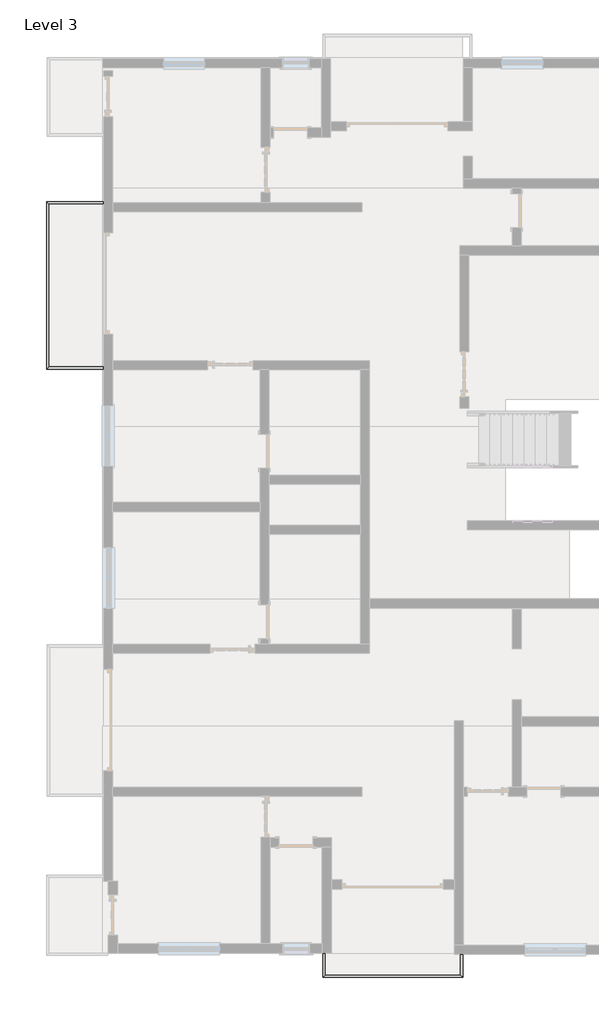
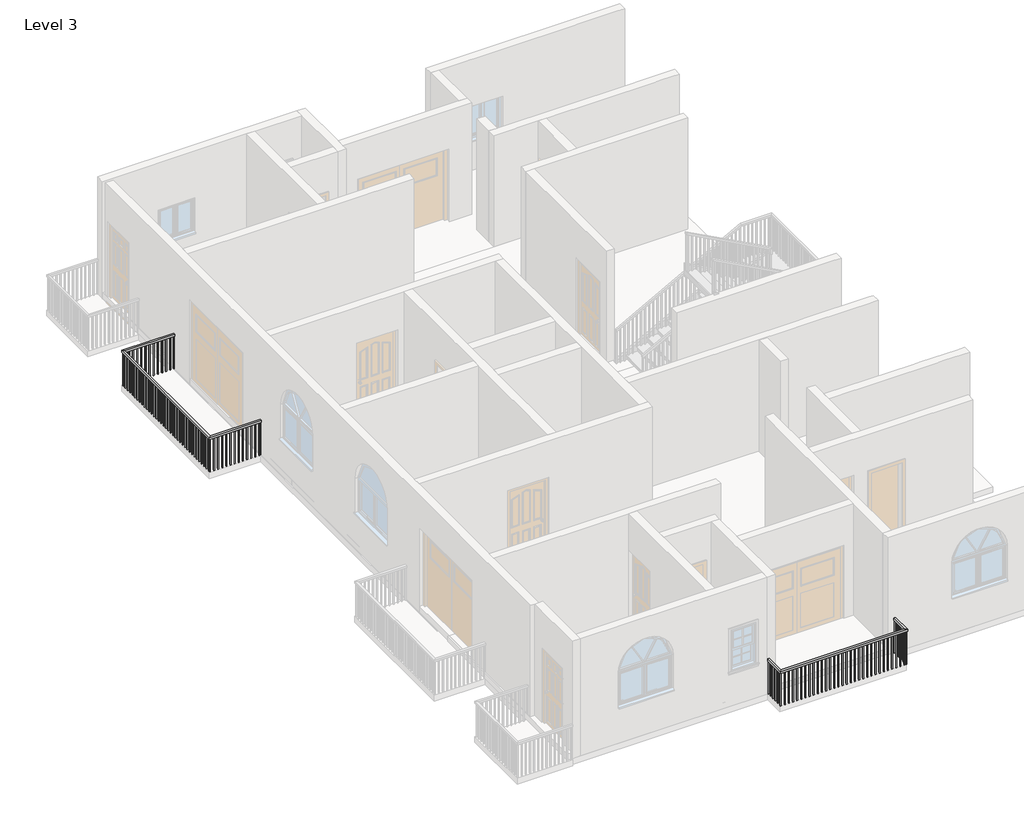
# One storey, part 4 of 7: 2 railings.
"""IFC4 building model written with IfcOpenShell, lengths in millimetres."""

from ifc_helpers import new_model, si_unit, frame, origin, place, context, project, spatial, polyline, outline, extrude, faceted_brep, element, save

model = new_model("IFC4")

# Units and contexts
model_context = context("Model", 3, world=origin())
ifc_project = project(units=[si_unit("LENGTHUNIT", "METRE", prefix="MILLI")], contexts=[model_context])

# Site, building, storey
site = spatial("IfcSite", under=ifc_project)
building = spatial("IfcBuilding", under=site)
storey = spatial("IfcBuildingStorey", under=building, Name="Level 3", Elevation=6096.0)

# Railings
placement = place(None, origin())
element("IfcRailing", 1, ObjectType="Handrail - Rectangular", at=placement, inside=storey, context=model_context, shape_type="SolidModel", body=[
    faceted_brep([(-1375.8109037, -10612.9037749, 7010.4), (-1375.8109037, -10612.9037749, 6959.6), (-1426.6109037, -10612.9037749, 6959.6), (-1426.6109037, -10612.9037749, 7010.4), (-1375.8109037, -11108.2037749, 7010.4), (-1375.8109037, -11108.2037749, 6959.6), (-1426.6109037, -11159.0037749, 6959.6), (-1426.6109037, -11159.0037749, 7010.4), (1659.4890963, -11108.2037749, 7010.4), (1659.4890963, -11108.2037749, 6959.6), (1710.2890963, -11159.0037749, 6959.6), (1710.2890963, -11159.0037749, 7010.4), (1659.4890963, -10638.3037749, 7010.4), (1710.2890963, -10638.3037749, 7010.4), (1710.2890963, -10638.3037749, 6959.6), (1659.4890963, -10638.3037749, 6959.6)], [[[0, 1, 2, 3]], [[1, 0, 4, 5]], [[2, 1, 5, 6]], [[3, 2, 6, 7]], [[0, 3, 7, 4]], [[5, 4, 8, 9]], [[6, 5, 9, 10]], [[7, 6, 10, 11]], [[4, 7, 11, 8]], [[12, 13, 14, 15]], [[9, 8, 12, 15]], [[10, 9, 15, 14]], [[11, 10, 14, 13]], [[8, 11, 13, 12]]]),
    extrude(outline(polyline([(1694.4140963, -10736.7287749), (1675.3640963, -10736.7287749), (1675.3640963, -10717.6787749), (1694.4140963, -10717.6787749), (1694.4140963, -10736.7287749)])), frame((0.0, 0.0, 6096.0), z_axis=(0.0, 0.0, 1.0), x_axis=(1.0, 0.0, 0.0)), (0.0, 0.0, 1.0), 863.6),
    extrude(outline(polyline([(1694.4140963, -10838.3287749), (1675.3640963, -10838.3287749), (1675.3640963, -10819.2787749), (1694.4140963, -10819.2787749), (1694.4140963, -10838.3287749)])), frame((0.0, 0.0, 6096.0), z_axis=(0.0, 0.0, 1.0), x_axis=(1.0, 0.0, 0.0)), (0.0, 0.0, 1.0), 863.6),
    extrude(outline(polyline([(1694.4140963, -10939.9287749), (1675.3640963, -10939.9287749), (1675.3640963, -10920.8787749), (1694.4140963, -10920.8787749), (1694.4140963, -10939.9287749)])), frame((0.0, 0.0, 6096.0), z_axis=(0.0, 0.0, 1.0), x_axis=(1.0, 0.0, 0.0)), (0.0, 0.0, 1.0), 863.6),
    extrude(outline(polyline([(1694.4140963, -11041.5287749), (1675.3640963, -11041.5287749), (1675.3640963, -11022.4787749), (1694.4140963, -11022.4787749), (1694.4140963, -11041.5287749)])), frame((0.0, 0.0, 6096.0), z_axis=(0.0, 0.0, 1.0), x_axis=(1.0, 0.0, 0.0)), (0.0, 0.0, 1.0), 863.6),
    extrude(outline(polyline([(1637.2640963, -11143.1287749), (1637.2640963, -11124.0787749), (1656.3140963, -11124.0787749), (1656.3140963, -11143.1287749), (1637.2640963, -11143.1287749)])), frame((0.0, 0.0, 6096.0), z_axis=(0.0, 0.0, 1.0), x_axis=(1.0, 0.0, 0.0)), (0.0, 0.0, 1.0), 863.6),
    extrude(outline(polyline([(1535.6640963, -11143.1287749), (1535.6640963, -11124.0787749), (1554.7140963, -11124.0787749), (1554.7140963, -11143.1287749), (1535.6640963, -11143.1287749)])), frame((0.0, 0.0, 6096.0), z_axis=(0.0, 0.0, 1.0), x_axis=(1.0, 0.0, 0.0)), (0.0, 0.0, 1.0), 863.6),
    extrude(outline(polyline([(1434.0640963, -11143.1287749), (1434.0640963, -11124.0787749), (1453.1140963, -11124.0787749), (1453.1140963, -11143.1287749), (1434.0640963, -11143.1287749)])), frame((0.0, 0.0, 6096.0), z_axis=(0.0, 0.0, 1.0), x_axis=(1.0, 0.0, 0.0)), (0.0, 0.0, 1.0), 863.6),
    extrude(outline(polyline([(1332.4640963, -11143.1287749), (1332.4640963, -11124.0787749), (1351.5140963, -11124.0787749), (1351.5140963, -11143.1287749), (1332.4640963, -11143.1287749)])), frame((0.0, 0.0, 6096.0), z_axis=(0.0, 0.0, 1.0), x_axis=(1.0, 0.0, 0.0)), (0.0, 0.0, 1.0), 863.6),
    extrude(outline(polyline([(1230.8640963, -11143.1287749), (1230.8640963, -11124.0787749), (1249.9140963, -11124.0787749), (1249.9140963, -11143.1287749), (1230.8640963, -11143.1287749)])), frame((0.0, 0.0, 6096.0), z_axis=(0.0, 0.0, 1.0), x_axis=(1.0, 0.0, 0.0)), (0.0, 0.0, 1.0), 863.6),
    extrude(outline(polyline([(1129.2640963, -11143.1287749), (1129.2640963, -11124.0787749), (1148.3140963, -11124.0787749), (1148.3140963, -11143.1287749), (1129.2640963, -11143.1287749)])), frame((0.0, 0.0, 6096.0), z_axis=(0.0, 0.0, 1.0), x_axis=(1.0, 0.0, 0.0)), (0.0, 0.0, 1.0), 863.6),
    extrude(outline(polyline([(1027.6640963, -11143.1287749), (1027.6640963, -11124.0787749), (1046.7140963, -11124.0787749), (1046.7140963, -11143.1287749), (1027.6640963, -11143.1287749)])), frame((0.0, 0.0, 6096.0), z_axis=(0.0, 0.0, 1.0), x_axis=(1.0, 0.0, 0.0)), (0.0, 0.0, 1.0), 863.6),
    extrude(outline(polyline([(926.0640963, -11143.1287749), (926.0640963, -11124.0787749), (945.1140963, -11124.0787749), (945.1140963, -11143.1287749), (926.0640963, -11143.1287749)])), frame((0.0, 0.0, 6096.0), z_axis=(0.0, 0.0, 1.0), x_axis=(1.0, 0.0, 0.0)), (0.0, 0.0, 1.0), 863.6),
    extrude(outline(polyline([(824.4640963, -11143.1287749), (824.4640963, -11124.0787749), (843.5140963, -11124.0787749), (843.5140963, -11143.1287749), (824.4640963, -11143.1287749)])), frame((0.0, 0.0, 6096.0), z_axis=(0.0, 0.0, 1.0), x_axis=(1.0, 0.0, 0.0)), (0.0, 0.0, 1.0), 863.6),
    extrude(outline(polyline([(722.8640963, -11143.1287749), (722.8640963, -11124.0787749), (741.9140963, -11124.0787749), (741.9140963, -11143.1287749), (722.8640963, -11143.1287749)])), frame((0.0, 0.0, 6096.0), z_axis=(0.0, 0.0, 1.0), x_axis=(1.0, 0.0, 0.0)), (0.0, 0.0, 1.0), 863.6),
    extrude(outline(polyline([(621.2640963, -11143.1287749), (621.2640963, -11124.0787749), (640.3140963, -11124.0787749), (640.3140963, -11143.1287749), (621.2640963, -11143.1287749)])), frame((0.0, 0.0, 6096.0), z_axis=(0.0, 0.0, 1.0), x_axis=(1.0, 0.0, 0.0)), (0.0, 0.0, 1.0), 863.6),
    extrude(outline(polyline([(519.6640963, -11143.1287749), (519.6640963, -11124.0787749), (538.7140963, -11124.0787749), (538.7140963, -11143.1287749), (519.6640963, -11143.1287749)])), frame((0.0, 0.0, 6096.0), z_axis=(0.0, 0.0, 1.0), x_axis=(1.0, 0.0, 0.0)), (0.0, 0.0, 1.0), 863.6),
    extrude(outline(polyline([(418.0640963, -11143.1287749), (418.0640963, -11124.0787749), (437.1140963, -11124.0787749), (437.1140963, -11143.1287749), (418.0640963, -11143.1287749)])), frame((0.0, 0.0, 6096.0), z_axis=(0.0, 0.0, 1.0), x_axis=(1.0, 0.0, 0.0)), (0.0, 0.0, 1.0), 863.6),
    extrude(outline(polyline([(316.4640963, -11143.1287749), (316.4640963, -11124.0787749), (335.5140963, -11124.0787749), (335.5140963, -11143.1287749), (316.4640963, -11143.1287749)])), frame((0.0, 0.0, 6096.0), z_axis=(0.0, 0.0, 1.0), x_axis=(1.0, 0.0, 0.0)), (0.0, 0.0, 1.0), 863.6),
    extrude(outline(polyline([(214.8640963, -11143.1287749), (214.8640963, -11124.0787749), (233.9140963, -11124.0787749), (233.9140963, -11143.1287749), (214.8640963, -11143.1287749)])), frame((0.0, 0.0, 6096.0), z_axis=(0.0, 0.0, 1.0), x_axis=(1.0, 0.0, 0.0)), (0.0, 0.0, 1.0), 863.6),
    extrude(outline(polyline([(113.2640963, -11143.1287749), (113.2640963, -11124.0787749), (132.3140963, -11124.0787749), (132.3140963, -11143.1287749), (113.2640963, -11143.1287749)])), frame((0.0, 0.0, 6096.0), z_axis=(0.0, 0.0, 1.0), x_axis=(1.0, 0.0, 0.0)), (0.0, 0.0, 1.0), 863.6),
    extrude(outline(polyline([(11.6640963, -11143.1287749), (11.6640963, -11124.0787749), (30.7140963, -11124.0787749), (30.7140963, -11143.1287749), (11.6640963, -11143.1287749)])), frame((0.0, 0.0, 6096.0), z_axis=(0.0, 0.0, 1.0), x_axis=(1.0, 0.0, 0.0)), (0.0, 0.0, 1.0), 863.6),
    extrude(outline(polyline([(-89.9359037, -11143.1287749), (-89.9359037, -11124.0787749), (-70.8859037, -11124.0787749), (-70.8859037, -11143.1287749), (-89.9359037, -11143.1287749)])), frame((0.0, 0.0, 6096.0), z_axis=(0.0, 0.0, 1.0), x_axis=(1.0, 0.0, 0.0)), (0.0, 0.0, 1.0), 863.6),
    extrude(outline(polyline([(-191.5359037, -11143.1287749), (-191.5359037, -11124.0787749), (-172.4859037, -11124.0787749), (-172.4859037, -11143.1287749), (-191.5359037, -11143.1287749)])), frame((0.0, 0.0, 6096.0), z_axis=(0.0, 0.0, 1.0), x_axis=(1.0, 0.0, 0.0)), (0.0, 0.0, 1.0), 863.6),
    extrude(outline(polyline([(-293.1359037, -11143.1287749), (-293.1359037, -11124.0787749), (-274.0859037, -11124.0787749), (-274.0859037, -11143.1287749), (-293.1359037, -11143.1287749)])), frame((0.0, 0.0, 6096.0), z_axis=(0.0, 0.0, 1.0), x_axis=(1.0, 0.0, 0.0)), (0.0, 0.0, 1.0), 863.6),
    extrude(outline(polyline([(-394.7359037, -11143.1287749), (-394.7359037, -11124.0787749), (-375.6859037, -11124.0787749), (-375.6859037, -11143.1287749), (-394.7359037, -11143.1287749)])), frame((0.0, 0.0, 6096.0), z_axis=(0.0, 0.0, 1.0), x_axis=(1.0, 0.0, 0.0)), (0.0, 0.0, 1.0), 863.6),
    extrude(outline(polyline([(-496.3359037, -11143.1287749), (-496.3359037, -11124.0787749), (-477.2859037, -11124.0787749), (-477.2859037, -11143.1287749), (-496.3359037, -11143.1287749)])), frame((0.0, 0.0, 6096.0), z_axis=(0.0, 0.0, 1.0), x_axis=(1.0, 0.0, 0.0)), (0.0, 0.0, 1.0), 863.6),
    extrude(outline(polyline([(-597.9359037, -11143.1287749), (-597.9359037, -11124.0787749), (-578.8859037, -11124.0787749), (-578.8859037, -11143.1287749), (-597.9359037, -11143.1287749)])), frame((0.0, 0.0, 6096.0), z_axis=(0.0, 0.0, 1.0), x_axis=(1.0, 0.0, 0.0)), (0.0, 0.0, 1.0), 863.6),
    extrude(outline(polyline([(-699.5359037, -11143.1287749), (-699.5359037, -11124.0787749), (-680.4859037, -11124.0787749), (-680.4859037, -11143.1287749), (-699.5359037, -11143.1287749)])), frame((0.0, 0.0, 6096.0), z_axis=(0.0, 0.0, 1.0), x_axis=(1.0, 0.0, 0.0)), (0.0, 0.0, 1.0), 863.6),
    extrude(outline(polyline([(-801.1359037, -11143.1287749), (-801.1359037, -11124.0787749), (-782.0859037, -11124.0787749), (-782.0859037, -11143.1287749), (-801.1359037, -11143.1287749)])), frame((0.0, 0.0, 6096.0), z_axis=(0.0, 0.0, 1.0), x_axis=(1.0, 0.0, 0.0)), (0.0, 0.0, 1.0), 863.6),
    extrude(outline(polyline([(-902.7359037, -11143.1287749), (-902.7359037, -11124.0787749), (-883.6859037, -11124.0787749), (-883.6859037, -11143.1287749), (-902.7359037, -11143.1287749)])), frame((0.0, 0.0, 6096.0), z_axis=(0.0, 0.0, 1.0), x_axis=(1.0, 0.0, 0.0)), (0.0, 0.0, 1.0), 863.6),
    extrude(outline(polyline([(-1004.3359037, -11143.1287749), (-1004.3359037, -11124.0787749), (-985.2859037, -11124.0787749), (-985.2859037, -11143.1287749), (-1004.3359037, -11143.1287749)])), frame((0.0, 0.0, 6096.0), z_axis=(0.0, 0.0, 1.0), x_axis=(1.0, 0.0, 0.0)), (0.0, 0.0, 1.0), 863.6),
    extrude(outline(polyline([(-1105.9359037, -11143.1287749), (-1105.9359037, -11124.0787749), (-1086.8859037, -11124.0787749), (-1086.8859037, -11143.1287749), (-1105.9359037, -11143.1287749)])), frame((0.0, 0.0, 6096.0), z_axis=(0.0, 0.0, 1.0), x_axis=(1.0, 0.0, 0.0)), (0.0, 0.0, 1.0), 863.6),
    extrude(outline(polyline([(-1207.5359037, -11143.1287749), (-1207.5359037, -11124.0787749), (-1188.4859037, -11124.0787749), (-1188.4859037, -11143.1287749), (-1207.5359037, -11143.1287749)])), frame((0.0, 0.0, 6096.0), z_axis=(0.0, 0.0, 1.0), x_axis=(1.0, 0.0, 0.0)), (0.0, 0.0, 1.0), 863.6),
    extrude(outline(polyline([(-1309.1359037, -11143.1287749), (-1309.1359037, -11124.0787749), (-1290.0859037, -11124.0787749), (-1290.0859037, -11143.1287749), (-1309.1359037, -11143.1287749)])), frame((0.0, 0.0, 6096.0), z_axis=(0.0, 0.0, 1.0), x_axis=(1.0, 0.0, 0.0)), (0.0, 0.0, 1.0), 863.6),
    extrude(outline(polyline([(-1410.7359037, -11111.3787749), (-1391.6859037, -11111.3787749), (-1391.6859037, -11130.4287749), (-1410.7359037, -11130.4287749), (-1410.7359037, -11111.3787749)])), frame((0.0, 0.0, 6096.0), z_axis=(0.0, 0.0, 1.0), x_axis=(1.0, 0.0, 0.0)), (0.0, 0.0, 1.0), 863.6),
    extrude(outline(polyline([(-1410.7359037, -11009.7787749), (-1391.6859037, -11009.7787749), (-1391.6859037, -11028.8287749), (-1410.7359037, -11028.8287749), (-1410.7359037, -11009.7787749)])), frame((0.0, 0.0, 6096.0), z_axis=(0.0, 0.0, 1.0), x_axis=(1.0, 0.0, 0.0)), (0.0, 0.0, 1.0), 863.6),
    extrude(outline(polyline([(-1410.7359037, -10908.1787749), (-1391.6859037, -10908.1787749), (-1391.6859037, -10927.2287749), (-1410.7359037, -10927.2287749), (-1410.7359037, -10908.1787749)])), frame((0.0, 0.0, 6096.0), z_axis=(0.0, 0.0, 1.0), x_axis=(1.0, 0.0, 0.0)), (0.0, 0.0, 1.0), 863.6),
    extrude(outline(polyline([(-1410.7359037, -10806.5787749), (-1391.6859037, -10806.5787749), (-1391.6859037, -10825.6287749), (-1410.7359037, -10825.6287749), (-1410.7359037, -10806.5787749)])), frame((0.0, 0.0, 6096.0), z_axis=(0.0, 0.0, 1.0), x_axis=(1.0, 0.0, 0.0)), (0.0, 0.0, 1.0), 863.6),
    extrude(outline(polyline([(-1410.7359037, -10704.9787749), (-1391.6859037, -10704.9787749), (-1391.6859037, -10724.0287749), (-1410.7359037, -10724.0287749), (-1410.7359037, -10704.9787749)])), frame((0.0, 0.0, 6096.0), z_axis=(0.0, 0.0, 1.0), x_axis=(1.0, 0.0, 0.0)), (0.0, 0.0, 1.0), 863.6),
    extrude(outline(polyline([(1675.3640963, -11143.1287749), (1675.3640963, -11124.0787749), (1694.4140963, -11124.0787749), (1694.4140963, -11143.1287749), (1675.3640963, -11143.1287749)])), frame((0.0, 0.0, 6096.0), z_axis=(0.0, 0.0, 1.0), x_axis=(1.0, 0.0, 0.0)), (0.0, 0.0, 1.0), 863.6),
    extrude(outline(polyline([(-1410.7359037, -11124.0787749), (-1391.6859037, -11124.0787749), (-1391.6859037, -11143.1287749), (-1410.7359037, -11143.1287749), (-1410.7359037, -11124.0787749)])), frame((0.0, 0.0, 6096.0), z_axis=(0.0, 0.0, 1.0), x_axis=(1.0, 0.0, 0.0)), (0.0, 0.0, 1.0), 863.6),
    extrude(outline(polyline([(1694.4140963, -10657.3537749), (1675.3640963, -10657.3537749), (1675.3640963, -10638.3037749), (1694.4140963, -10638.3037749), (1694.4140963, -10657.3537749)])), frame((0.0, 0.0, 6096.0), z_axis=(0.0, 0.0, 1.0), x_axis=(1.0, 0.0, 0.0)), (0.0, 0.0, 1.0), 863.6),
    extrude(outline(polyline([(-1410.7359037, -10612.9037749), (-1391.6859037, -10612.9037749), (-1391.6859037, -10631.9537749), (-1410.7359037, -10631.9537749), (-1410.7359037, -10612.9037749)])), frame((0.0, 0.0, 6096.0), z_axis=(0.0, 0.0, 1.0), x_axis=(1.0, 0.0, 0.0)), (0.0, 0.0, 1.0), 863.6),
])
element("IfcRailing", 2, ObjectType="Handrail - Rectangular", at=placement, inside=storey, context=model_context, shape_type="SolidModel", body=[
    faceted_brep([(-6330.8013636, 6151.0962251, 7010.4), (-6330.8013636, 6151.0962251, 6959.6), (-6330.8013636, 6201.8962251, 6959.6), (-6330.8013636, 6201.8962251, 7010.4), (-7563.8859037, 6151.0962251, 7010.4), (-7563.8859037, 6151.0962251, 6959.6), (-7614.6859037, 6201.8962251, 6959.6), (-7614.6859037, 6201.8962251, 7010.4), (-7563.8859037, 2506.1962251, 7010.4), (-7563.8859037, 2506.1962251, 6959.6), (-7614.6859037, 2455.3962251, 6959.6), (-7614.6859037, 2455.3962251, 7010.4), (-6330.8013636, 2506.1962251, 7010.4), (-6330.8013636, 2455.3962251, 7010.4), (-6330.8013636, 2455.3962251, 6959.6), (-6330.8013636, 2506.1962251, 6959.6)], [[[0, 1, 2, 3]], [[1, 0, 4, 5]], [[2, 1, 5, 6]], [[3, 2, 6, 7]], [[0, 3, 7, 4]], [[5, 4, 8, 9]], [[6, 5, 9, 10]], [[7, 6, 10, 11]], [[4, 7, 11, 8]], [[12, 13, 14, 15]], [[9, 8, 12, 15]], [[10, 9, 15, 14]], [[11, 10, 14, 13]], [[8, 11, 13, 12]]]),
    extrude(outline(polyline([(-6379.6109037, 2471.2712251), (-6379.6109037, 2490.3212251), (-6360.5609037, 2490.3212251), (-6360.5609037, 2471.2712251), (-6379.6109037, 2471.2712251)])), frame((0.0, 0.0, 6096.0), z_axis=(0.0, 0.0, 1.0), x_axis=(1.0, 0.0, 0.0)), (0.0, 0.0, 1.0), 863.6),
    extrude(outline(polyline([(-6481.2109037, 2471.2712251), (-6481.2109037, 2490.3212251), (-6462.1609037, 2490.3212251), (-6462.1609037, 2471.2712251), (-6481.2109037, 2471.2712251)])), frame((0.0, 0.0, 6096.0), z_axis=(0.0, 0.0, 1.0), x_axis=(1.0, 0.0, 0.0)), (0.0, 0.0, 1.0), 863.6),
    extrude(outline(polyline([(-6582.8109037, 2471.2712251), (-6582.8109037, 2490.3212251), (-6563.7609037, 2490.3212251), (-6563.7609037, 2471.2712251), (-6582.8109037, 2471.2712251)])), frame((0.0, 0.0, 6096.0), z_axis=(0.0, 0.0, 1.0), x_axis=(1.0, 0.0, 0.0)), (0.0, 0.0, 1.0), 863.6),
    extrude(outline(polyline([(-6684.4109037, 2471.2712251), (-6684.4109037, 2490.3212251), (-6665.3609037, 2490.3212251), (-6665.3609037, 2471.2712251), (-6684.4109037, 2471.2712251)])), frame((0.0, 0.0, 6096.0), z_axis=(0.0, 0.0, 1.0), x_axis=(1.0, 0.0, 0.0)), (0.0, 0.0, 1.0), 863.6),
    extrude(outline(polyline([(-6786.0109037, 2471.2712251), (-6786.0109037, 2490.3212251), (-6766.9609037, 2490.3212251), (-6766.9609037, 2471.2712251), (-6786.0109037, 2471.2712251)])), frame((0.0, 0.0, 6096.0), z_axis=(0.0, 0.0, 1.0), x_axis=(1.0, 0.0, 0.0)), (0.0, 0.0, 1.0), 863.6),
    extrude(outline(polyline([(-6887.6109037, 2471.2712251), (-6887.6109037, 2490.3212251), (-6868.5609037, 2490.3212251), (-6868.5609037, 2471.2712251), (-6887.6109037, 2471.2712251)])), frame((0.0, 0.0, 6096.0), z_axis=(0.0, 0.0, 1.0), x_axis=(1.0, 0.0, 0.0)), (0.0, 0.0, 1.0), 863.6),
    extrude(outline(polyline([(-6989.2109037, 2471.2712251), (-6989.2109037, 2490.3212251), (-6970.1609037, 2490.3212251), (-6970.1609037, 2471.2712251), (-6989.2109037, 2471.2712251)])), frame((0.0, 0.0, 6096.0), z_axis=(0.0, 0.0, 1.0), x_axis=(1.0, 0.0, 0.0)), (0.0, 0.0, 1.0), 863.6),
    extrude(outline(polyline([(-7090.8109037, 2471.2712251), (-7090.8109037, 2490.3212251), (-7071.7609037, 2490.3212251), (-7071.7609037, 2471.2712251), (-7090.8109037, 2471.2712251)])), frame((0.0, 0.0, 6096.0), z_axis=(0.0, 0.0, 1.0), x_axis=(1.0, 0.0, 0.0)), (0.0, 0.0, 1.0), 863.6),
    extrude(outline(polyline([(-7192.4109037, 2471.2712251), (-7192.4109037, 2490.3212251), (-7173.3609037, 2490.3212251), (-7173.3609037, 2471.2712251), (-7192.4109037, 2471.2712251)])), frame((0.0, 0.0, 6096.0), z_axis=(0.0, 0.0, 1.0), x_axis=(1.0, 0.0, 0.0)), (0.0, 0.0, 1.0), 863.6),
    extrude(outline(polyline([(-7294.0109037, 2471.2712251), (-7294.0109037, 2490.3212251), (-7274.9609037, 2490.3212251), (-7274.9609037, 2471.2712251), (-7294.0109037, 2471.2712251)])), frame((0.0, 0.0, 6096.0), z_axis=(0.0, 0.0, 1.0), x_axis=(1.0, 0.0, 0.0)), (0.0, 0.0, 1.0), 863.6),
    extrude(outline(polyline([(-7395.6109037, 2471.2712251), (-7395.6109037, 2490.3212251), (-7376.5609037, 2490.3212251), (-7376.5609037, 2471.2712251), (-7395.6109037, 2471.2712251)])), frame((0.0, 0.0, 6096.0), z_axis=(0.0, 0.0, 1.0), x_axis=(1.0, 0.0, 0.0)), (0.0, 0.0, 1.0), 863.6),
    extrude(outline(polyline([(-7497.2109037, 2471.2712251), (-7497.2109037, 2490.3212251), (-7478.1609037, 2490.3212251), (-7478.1609037, 2471.2712251), (-7497.2109037, 2471.2712251)])), frame((0.0, 0.0, 6096.0), z_axis=(0.0, 0.0, 1.0), x_axis=(1.0, 0.0, 0.0)), (0.0, 0.0, 1.0), 863.6),
    extrude(outline(polyline([(-7598.8109037, 2528.4212251), (-7579.7609037, 2528.4212251), (-7579.7609037, 2509.3712251), (-7598.8109037, 2509.3712251), (-7598.8109037, 2528.4212251)])), frame((0.0, 0.0, 6096.0), z_axis=(0.0, 0.0, 1.0), x_axis=(1.0, 0.0, 0.0)), (0.0, 0.0, 1.0), 863.6),
    extrude(outline(polyline([(-7598.8109037, 2630.0212251), (-7579.7609037, 2630.0212251), (-7579.7609037, 2610.9712251), (-7598.8109037, 2610.9712251), (-7598.8109037, 2630.0212251)])), frame((0.0, 0.0, 6096.0), z_axis=(0.0, 0.0, 1.0), x_axis=(1.0, 0.0, 0.0)), (0.0, 0.0, 1.0), 863.6),
    extrude(outline(polyline([(-7598.8109037, 2731.6212251), (-7579.7609037, 2731.6212251), (-7579.7609037, 2712.5712251), (-7598.8109037, 2712.5712251), (-7598.8109037, 2731.6212251)])), frame((0.0, 0.0, 6096.0), z_axis=(0.0, 0.0, 1.0), x_axis=(1.0, 0.0, 0.0)), (0.0, 0.0, 1.0), 863.6),
    extrude(outline(polyline([(-7598.8109037, 2833.2212251), (-7579.7609037, 2833.2212251), (-7579.7609037, 2814.1712251), (-7598.8109037, 2814.1712251), (-7598.8109037, 2833.2212251)])), frame((0.0, 0.0, 6096.0), z_axis=(0.0, 0.0, 1.0), x_axis=(1.0, 0.0, 0.0)), (0.0, 0.0, 1.0), 863.6),
    extrude(outline(polyline([(-7598.8109037, 2934.8212251), (-7579.7609037, 2934.8212251), (-7579.7609037, 2915.7712251), (-7598.8109037, 2915.7712251), (-7598.8109037, 2934.8212251)])), frame((0.0, 0.0, 6096.0), z_axis=(0.0, 0.0, 1.0), x_axis=(1.0, 0.0, 0.0)), (0.0, 0.0, 1.0), 863.6),
    extrude(outline(polyline([(-7598.8109037, 3036.4212251), (-7579.7609037, 3036.4212251), (-7579.7609037, 3017.3712251), (-7598.8109037, 3017.3712251), (-7598.8109037, 3036.4212251)])), frame((0.0, 0.0, 6096.0), z_axis=(0.0, 0.0, 1.0), x_axis=(1.0, 0.0, 0.0)), (0.0, 0.0, 1.0), 863.6),
    extrude(outline(polyline([(-7598.8109037, 3138.0212251), (-7579.7609037, 3138.0212251), (-7579.7609037, 3118.9712251), (-7598.8109037, 3118.9712251), (-7598.8109037, 3138.0212251)])), frame((0.0, 0.0, 6096.0), z_axis=(0.0, 0.0, 1.0), x_axis=(1.0, 0.0, 0.0)), (0.0, 0.0, 1.0), 863.6),
    extrude(outline(polyline([(-7598.8109037, 3239.6212251), (-7579.7609037, 3239.6212251), (-7579.7609037, 3220.5712251), (-7598.8109037, 3220.5712251), (-7598.8109037, 3239.6212251)])), frame((0.0, 0.0, 6096.0), z_axis=(0.0, 0.0, 1.0), x_axis=(1.0, 0.0, 0.0)), (0.0, 0.0, 1.0), 863.6),
    extrude(outline(polyline([(-7598.8109037, 3341.2212251), (-7579.7609037, 3341.2212251), (-7579.7609037, 3322.1712251), (-7598.8109037, 3322.1712251), (-7598.8109037, 3341.2212251)])), frame((0.0, 0.0, 6096.0), z_axis=(0.0, 0.0, 1.0), x_axis=(1.0, 0.0, 0.0)), (0.0, 0.0, 1.0), 863.6),
    extrude(outline(polyline([(-7598.8109037, 3442.8212251), (-7579.7609037, 3442.8212251), (-7579.7609037, 3423.7712251), (-7598.8109037, 3423.7712251), (-7598.8109037, 3442.8212251)])), frame((0.0, 0.0, 6096.0), z_axis=(0.0, 0.0, 1.0), x_axis=(1.0, 0.0, 0.0)), (0.0, 0.0, 1.0), 863.6),
    extrude(outline(polyline([(-7598.8109037, 3544.4212251), (-7579.7609037, 3544.4212251), (-7579.7609037, 3525.3712251), (-7598.8109037, 3525.3712251), (-7598.8109037, 3544.4212251)])), frame((0.0, 0.0, 6096.0), z_axis=(0.0, 0.0, 1.0), x_axis=(1.0, 0.0, 0.0)), (0.0, 0.0, 1.0), 863.6),
    extrude(outline(polyline([(-7598.8109037, 3646.0212251), (-7579.7609037, 3646.0212251), (-7579.7609037, 3626.9712251), (-7598.8109037, 3626.9712251), (-7598.8109037, 3646.0212251)])), frame((0.0, 0.0, 6096.0), z_axis=(0.0, 0.0, 1.0), x_axis=(1.0, 0.0, 0.0)), (0.0, 0.0, 1.0), 863.6),
    extrude(outline(polyline([(-7598.8109037, 3747.6212251), (-7579.7609037, 3747.6212251), (-7579.7609037, 3728.5712251), (-7598.8109037, 3728.5712251), (-7598.8109037, 3747.6212251)])), frame((0.0, 0.0, 6096.0), z_axis=(0.0, 0.0, 1.0), x_axis=(1.0, 0.0, 0.0)), (0.0, 0.0, 1.0), 863.6),
    extrude(outline(polyline([(-7598.8109037, 3849.2212251), (-7579.7609037, 3849.2212251), (-7579.7609037, 3830.1712251), (-7598.8109037, 3830.1712251), (-7598.8109037, 3849.2212251)])), frame((0.0, 0.0, 6096.0), z_axis=(0.0, 0.0, 1.0), x_axis=(1.0, 0.0, 0.0)), (0.0, 0.0, 1.0), 863.6),
    extrude(outline(polyline([(-7598.8109037, 3950.8212251), (-7579.7609037, 3950.8212251), (-7579.7609037, 3931.7712251), (-7598.8109037, 3931.7712251), (-7598.8109037, 3950.8212251)])), frame((0.0, 0.0, 6096.0), z_axis=(0.0, 0.0, 1.0), x_axis=(1.0, 0.0, 0.0)), (0.0, 0.0, 1.0), 863.6),
    extrude(outline(polyline([(-7598.8109037, 4052.4212251), (-7579.7609037, 4052.4212251), (-7579.7609037, 4033.3712251), (-7598.8109037, 4033.3712251), (-7598.8109037, 4052.4212251)])), frame((0.0, 0.0, 6096.0), z_axis=(0.0, 0.0, 1.0), x_axis=(1.0, 0.0, 0.0)), (0.0, 0.0, 1.0), 863.6),
    extrude(outline(polyline([(-7598.8109037, 4154.0212251), (-7579.7609037, 4154.0212251), (-7579.7609037, 4134.9712251), (-7598.8109037, 4134.9712251), (-7598.8109037, 4154.0212251)])), frame((0.0, 0.0, 6096.0), z_axis=(0.0, 0.0, 1.0), x_axis=(1.0, 0.0, 0.0)), (0.0, 0.0, 1.0), 863.6),
    extrude(outline(polyline([(-7598.8109037, 4255.6212251), (-7579.7609037, 4255.6212251), (-7579.7609037, 4236.5712251), (-7598.8109037, 4236.5712251), (-7598.8109037, 4255.6212251)])), frame((0.0, 0.0, 6096.0), z_axis=(0.0, 0.0, 1.0), x_axis=(1.0, 0.0, 0.0)), (0.0, 0.0, 1.0), 863.6),
    extrude(outline(polyline([(-7598.8109037, 4357.2212251), (-7579.7609037, 4357.2212251), (-7579.7609037, 4338.1712251), (-7598.8109037, 4338.1712251), (-7598.8109037, 4357.2212251)])), frame((0.0, 0.0, 6096.0), z_axis=(0.0, 0.0, 1.0), x_axis=(1.0, 0.0, 0.0)), (0.0, 0.0, 1.0), 863.6),
    extrude(outline(polyline([(-7598.8109037, 4458.8212251), (-7579.7609037, 4458.8212251), (-7579.7609037, 4439.7712251), (-7598.8109037, 4439.7712251), (-7598.8109037, 4458.8212251)])), frame((0.0, 0.0, 6096.0), z_axis=(0.0, 0.0, 1.0), x_axis=(1.0, 0.0, 0.0)), (0.0, 0.0, 1.0), 863.6),
    extrude(outline(polyline([(-7598.8109037, 4560.4212251), (-7579.7609037, 4560.4212251), (-7579.7609037, 4541.3712251), (-7598.8109037, 4541.3712251), (-7598.8109037, 4560.4212251)])), frame((0.0, 0.0, 6096.0), z_axis=(0.0, 0.0, 1.0), x_axis=(1.0, 0.0, 0.0)), (0.0, 0.0, 1.0), 863.6),
    extrude(outline(polyline([(-7598.8109037, 4662.0212251), (-7579.7609037, 4662.0212251), (-7579.7609037, 4642.9712251), (-7598.8109037, 4642.9712251), (-7598.8109037, 4662.0212251)])), frame((0.0, 0.0, 6096.0), z_axis=(0.0, 0.0, 1.0), x_axis=(1.0, 0.0, 0.0)), (0.0, 0.0, 1.0), 863.6),
    extrude(outline(polyline([(-7598.8109037, 4763.6212251), (-7579.7609037, 4763.6212251), (-7579.7609037, 4744.5712251), (-7598.8109037, 4744.5712251), (-7598.8109037, 4763.6212251)])), frame((0.0, 0.0, 6096.0), z_axis=(0.0, 0.0, 1.0), x_axis=(1.0, 0.0, 0.0)), (0.0, 0.0, 1.0), 863.6),
    extrude(outline(polyline([(-7598.8109037, 4865.2212251), (-7579.7609037, 4865.2212251), (-7579.7609037, 4846.1712251), (-7598.8109037, 4846.1712251), (-7598.8109037, 4865.2212251)])), frame((0.0, 0.0, 6096.0), z_axis=(0.0, 0.0, 1.0), x_axis=(1.0, 0.0, 0.0)), (0.0, 0.0, 1.0), 863.6),
    extrude(outline(polyline([(-7598.8109037, 4966.8212251), (-7579.7609037, 4966.8212251), (-7579.7609037, 4947.7712251), (-7598.8109037, 4947.7712251), (-7598.8109037, 4966.8212251)])), frame((0.0, 0.0, 6096.0), z_axis=(0.0, 0.0, 1.0), x_axis=(1.0, 0.0, 0.0)), (0.0, 0.0, 1.0), 863.6),
    extrude(outline(polyline([(-7598.8109037, 5068.4212251), (-7579.7609037, 5068.4212251), (-7579.7609037, 5049.3712251), (-7598.8109037, 5049.3712251), (-7598.8109037, 5068.4212251)])), frame((0.0, 0.0, 6096.0), z_axis=(0.0, 0.0, 1.0), x_axis=(1.0, 0.0, 0.0)), (0.0, 0.0, 1.0), 863.6),
    extrude(outline(polyline([(-7598.8109037, 5170.0212251), (-7579.7609037, 5170.0212251), (-7579.7609037, 5150.9712251), (-7598.8109037, 5150.9712251), (-7598.8109037, 5170.0212251)])), frame((0.0, 0.0, 6096.0), z_axis=(0.0, 0.0, 1.0), x_axis=(1.0, 0.0, 0.0)), (0.0, 0.0, 1.0), 863.6),
    extrude(outline(polyline([(-7598.8109037, 5271.6212251), (-7579.7609037, 5271.6212251), (-7579.7609037, 5252.5712251), (-7598.8109037, 5252.5712251), (-7598.8109037, 5271.6212251)])), frame((0.0, 0.0, 6096.0), z_axis=(0.0, 0.0, 1.0), x_axis=(1.0, 0.0, 0.0)), (0.0, 0.0, 1.0), 863.6),
    extrude(outline(polyline([(-7598.8109037, 5373.2212251), (-7579.7609037, 5373.2212251), (-7579.7609037, 5354.1712251), (-7598.8109037, 5354.1712251), (-7598.8109037, 5373.2212251)])), frame((0.0, 0.0, 6096.0), z_axis=(0.0, 0.0, 1.0), x_axis=(1.0, 0.0, 0.0)), (0.0, 0.0, 1.0), 863.6),
    extrude(outline(polyline([(-7598.8109037, 5474.8212251), (-7579.7609037, 5474.8212251), (-7579.7609037, 5455.7712251), (-7598.8109037, 5455.7712251), (-7598.8109037, 5474.8212251)])), frame((0.0, 0.0, 6096.0), z_axis=(0.0, 0.0, 1.0), x_axis=(1.0, 0.0, 0.0)), (0.0, 0.0, 1.0), 863.6),
    extrude(outline(polyline([(-7598.8109037, 5576.4212251), (-7579.7609037, 5576.4212251), (-7579.7609037, 5557.3712251), (-7598.8109037, 5557.3712251), (-7598.8109037, 5576.4212251)])), frame((0.0, 0.0, 6096.0), z_axis=(0.0, 0.0, 1.0), x_axis=(1.0, 0.0, 0.0)), (0.0, 0.0, 1.0), 863.6),
    extrude(outline(polyline([(-7598.8109037, 5678.0212251), (-7579.7609037, 5678.0212251), (-7579.7609037, 5658.9712251), (-7598.8109037, 5658.9712251), (-7598.8109037, 5678.0212251)])), frame((0.0, 0.0, 6096.0), z_axis=(0.0, 0.0, 1.0), x_axis=(1.0, 0.0, 0.0)), (0.0, 0.0, 1.0), 863.6),
    extrude(outline(polyline([(-7598.8109037, 5779.6212251), (-7579.7609037, 5779.6212251), (-7579.7609037, 5760.5712251), (-7598.8109037, 5760.5712251), (-7598.8109037, 5779.6212251)])), frame((0.0, 0.0, 6096.0), z_axis=(0.0, 0.0, 1.0), x_axis=(1.0, 0.0, 0.0)), (0.0, 0.0, 1.0), 863.6),
    extrude(outline(polyline([(-7598.8109037, 5881.2212251), (-7579.7609037, 5881.2212251), (-7579.7609037, 5862.1712251), (-7598.8109037, 5862.1712251), (-7598.8109037, 5881.2212251)])), frame((0.0, 0.0, 6096.0), z_axis=(0.0, 0.0, 1.0), x_axis=(1.0, 0.0, 0.0)), (0.0, 0.0, 1.0), 863.6),
    extrude(outline(polyline([(-7598.8109037, 5982.8212251), (-7579.7609037, 5982.8212251), (-7579.7609037, 5963.7712251), (-7598.8109037, 5963.7712251), (-7598.8109037, 5982.8212251)])), frame((0.0, 0.0, 6096.0), z_axis=(0.0, 0.0, 1.0), x_axis=(1.0, 0.0, 0.0)), (0.0, 0.0, 1.0), 863.6),
    extrude(outline(polyline([(-7598.8109037, 6084.4212251), (-7579.7609037, 6084.4212251), (-7579.7609037, 6065.3712251), (-7598.8109037, 6065.3712251), (-7598.8109037, 6084.4212251)])), frame((0.0, 0.0, 6096.0), z_axis=(0.0, 0.0, 1.0), x_axis=(1.0, 0.0, 0.0)), (0.0, 0.0, 1.0), 863.6),
    extrude(outline(polyline([(-7540.4763636, 6186.0212251), (-7540.4763636, 6166.9712251), (-7559.5263636, 6166.9712251), (-7559.5263636, 6186.0212251), (-7540.4763636, 6186.0212251)])), frame((0.0, 0.0, 6096.0), z_axis=(0.0, 0.0, 1.0), x_axis=(1.0, 0.0, 0.0)), (0.0, 0.0, 1.0), 863.6),
    extrude(outline(polyline([(-7438.8763636, 6186.0212251), (-7438.8763636, 6166.9712251), (-7457.9263636, 6166.9712251), (-7457.9263636, 6186.0212251), (-7438.8763636, 6186.0212251)])), frame((0.0, 0.0, 6096.0), z_axis=(0.0, 0.0, 1.0), x_axis=(1.0, 0.0, 0.0)), (0.0, 0.0, 1.0), 863.6),
    extrude(outline(polyline([(-7337.2763636, 6186.0212251), (-7337.2763636, 6166.9712251), (-7356.3263636, 6166.9712251), (-7356.3263636, 6186.0212251), (-7337.2763636, 6186.0212251)])), frame((0.0, 0.0, 6096.0), z_axis=(0.0, 0.0, 1.0), x_axis=(1.0, 0.0, 0.0)), (0.0, 0.0, 1.0), 863.6),
    extrude(outline(polyline([(-7235.6763636, 6186.0212251), (-7235.6763636, 6166.9712251), (-7254.7263636, 6166.9712251), (-7254.7263636, 6186.0212251), (-7235.6763636, 6186.0212251)])), frame((0.0, 0.0, 6096.0), z_axis=(0.0, 0.0, 1.0), x_axis=(1.0, 0.0, 0.0)), (0.0, 0.0, 1.0), 863.6),
    extrude(outline(polyline([(-7134.0763636, 6186.0212251), (-7134.0763636, 6166.9712251), (-7153.1263636, 6166.9712251), (-7153.1263636, 6186.0212251), (-7134.0763636, 6186.0212251)])), frame((0.0, 0.0, 6096.0), z_axis=(0.0, 0.0, 1.0), x_axis=(1.0, 0.0, 0.0)), (0.0, 0.0, 1.0), 863.6),
    extrude(outline(polyline([(-7032.4763636, 6186.0212251), (-7032.4763636, 6166.9712251), (-7051.5263636, 6166.9712251), (-7051.5263636, 6186.0212251), (-7032.4763636, 6186.0212251)])), frame((0.0, 0.0, 6096.0), z_axis=(0.0, 0.0, 1.0), x_axis=(1.0, 0.0, 0.0)), (0.0, 0.0, 1.0), 863.6),
    extrude(outline(polyline([(-6930.8763636, 6186.0212251), (-6930.8763636, 6166.9712251), (-6949.9263636, 6166.9712251), (-6949.9263636, 6186.0212251), (-6930.8763636, 6186.0212251)])), frame((0.0, 0.0, 6096.0), z_axis=(0.0, 0.0, 1.0), x_axis=(1.0, 0.0, 0.0)), (0.0, 0.0, 1.0), 863.6),
    extrude(outline(polyline([(-6829.2763636, 6186.0212251), (-6829.2763636, 6166.9712251), (-6848.3263636, 6166.9712251), (-6848.3263636, 6186.0212251), (-6829.2763636, 6186.0212251)])), frame((0.0, 0.0, 6096.0), z_axis=(0.0, 0.0, 1.0), x_axis=(1.0, 0.0, 0.0)), (0.0, 0.0, 1.0), 863.6),
    extrude(outline(polyline([(-6727.6763636, 6186.0212251), (-6727.6763636, 6166.9712251), (-6746.7263636, 6166.9712251), (-6746.7263636, 6186.0212251), (-6727.6763636, 6186.0212251)])), frame((0.0, 0.0, 6096.0), z_axis=(0.0, 0.0, 1.0), x_axis=(1.0, 0.0, 0.0)), (0.0, 0.0, 1.0), 863.6),
    extrude(outline(polyline([(-6626.0763636, 6186.0212251), (-6626.0763636, 6166.9712251), (-6645.1263636, 6166.9712251), (-6645.1263636, 6186.0212251), (-6626.0763636, 6186.0212251)])), frame((0.0, 0.0, 6096.0), z_axis=(0.0, 0.0, 1.0), x_axis=(1.0, 0.0, 0.0)), (0.0, 0.0, 1.0), 863.6),
    extrude(outline(polyline([(-6524.4763636, 6186.0212251), (-6524.4763636, 6166.9712251), (-6543.5263636, 6166.9712251), (-6543.5263636, 6186.0212251), (-6524.4763636, 6186.0212251)])), frame((0.0, 0.0, 6096.0), z_axis=(0.0, 0.0, 1.0), x_axis=(1.0, 0.0, 0.0)), (0.0, 0.0, 1.0), 863.6),
    extrude(outline(polyline([(-6422.8763636, 6186.0212251), (-6422.8763636, 6166.9712251), (-6441.9263636, 6166.9712251), (-6441.9263636, 6186.0212251), (-6422.8763636, 6186.0212251)])), frame((0.0, 0.0, 6096.0), z_axis=(0.0, 0.0, 1.0), x_axis=(1.0, 0.0, 0.0)), (0.0, 0.0, 1.0), 863.6),
    extrude(outline(polyline([(-7598.8109037, 2490.3212251), (-7579.7609037, 2490.3212251), (-7579.7609037, 2471.2712251), (-7598.8109037, 2471.2712251), (-7598.8109037, 2490.3212251)])), frame((0.0, 0.0, 6096.0), z_axis=(0.0, 0.0, 1.0), x_axis=(1.0, 0.0, 0.0)), (0.0, 0.0, 1.0), 863.6),
    extrude(outline(polyline([(-7579.7609037, 6186.0212251), (-7579.7609037, 6166.9712251), (-7598.8109037, 6166.9712251), (-7598.8109037, 6186.0212251), (-7579.7609037, 6186.0212251)])), frame((0.0, 0.0, 6096.0), z_axis=(0.0, 0.0, 1.0), x_axis=(1.0, 0.0, 0.0)), (0.0, 0.0, 1.0), 863.6),
    extrude(outline(polyline([(-6349.8513636, 2471.2712251), (-6349.8513636, 2490.3212251), (-6330.8013636, 2490.3212251), (-6330.8013636, 2471.2712251), (-6349.8513636, 2471.2712251)])), frame((0.0, 0.0, 6096.0), z_axis=(0.0, 0.0, 1.0), x_axis=(1.0, 0.0, 0.0)), (0.0, 0.0, 1.0), 863.6),
    extrude(outline(polyline([(-6330.8013636, 6186.0212251), (-6330.8013636, 6166.9712251), (-6349.8513636, 6166.9712251), (-6349.8513636, 6186.0212251), (-6330.8013636, 6186.0212251)])), frame((0.0, 0.0, 6096.0), z_axis=(0.0, 0.0, 1.0), x_axis=(1.0, 0.0, 0.0)), (0.0, 0.0, 1.0), 863.6),
])

save(model, "model.ifc")

# Revit data of these elements
# Type "Handrail - Rectangular"
#   Assembly Code = "C2010400"
#   built-in parameter 1008612 = 0.0416667 (stored number, unit not read)
#   built-in parameter 1008611 = 0.0416667 (stored number, unit not read)
#   built-in parameter 1008609 = 0.333333 (stored number, unit not read)
#   built-in parameter 1008604 = 0.166667 (stored number, unit not read)
#   built-in parameter 1008603 = 0.166667 (stored number, unit not read)
#   Railing Height = 3' - 0"
#   built-in parameter 1008630 = 2
#   built-in parameter 1008610 = 2
#   built-in parameter 1008618 = Baluster - Square : 3/4"
# Elements 1, 2 (IfcRailing, "Handrail - Rectangular")
#   Phase Created = New Construction
